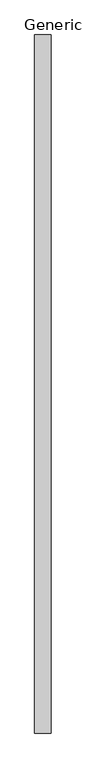
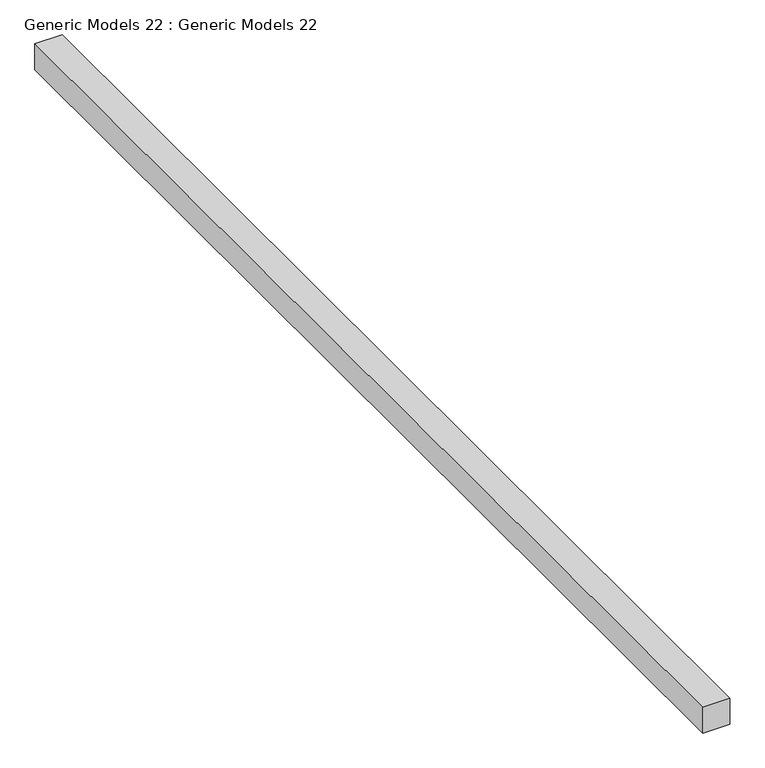
"""IFC4 building model written with IfcOpenShell, lengths in millimetres: proxy geometry, Generic Models 22 : Generic Models 22."""

from ifc_helpers import new_model, si_unit, frame, origin, place, context, project, spatial, polyline, outline, extrude, source, transform, mapped, element, save


def generic_models_22_generic_models_22_0e0807fa(model_context):
    return source(origin(), model_context, "Body", "SweptSolid", [
        extrude(outline(polyline([(-15479.838074, -6025.4275045), (-15479.838074, 6977.5785374), (-15175.038074, 6977.5785374), (-15175.038074, -6025.4275045), (-15479.838074, -6025.4275045)])), frame((0.0, 0.0, 5791.2), z_axis=(0.0, 0.0, 1.0), x_axis=(1.0, 0.0, 0.0)), (0.0, 0.0, 1.0), 304.8),
    ])


if __name__ == "__main__":
    model = new_model("IFC4")
    model_context = context("Model", 3, world=origin())
    ifc_project = project(units=[si_unit("LENGTHUNIT", "METRE", prefix="MILLI")], contexts=[model_context])
    site = spatial("IfcSite", under=ifc_project)
    building = spatial("IfcBuilding", under=site)
    placement = place(None, origin())
    generic_models_22_generic_models_22_shape = generic_models_22_generic_models_22_0e0807fa(model_context)
    element("IfcBuildingElementProxy", 1, Name="Generic Models 22 : Generic Models 22", ObjectType="Generic Models 22 : Generic Models 22", at=placement, inside=building, context=model_context, shape_type="MappedRepresentation", body=[
        mapped(generic_models_22_generic_models_22_shape, transform((0.0, 0.0, 0.0), x_axis=(1.0, 0.0, 0.0), y_axis=(0.0, 1.0, 0.0), z_axis=(0.0, 0.0, 1.0))),
    ])
    save(model, "model.ifc")
